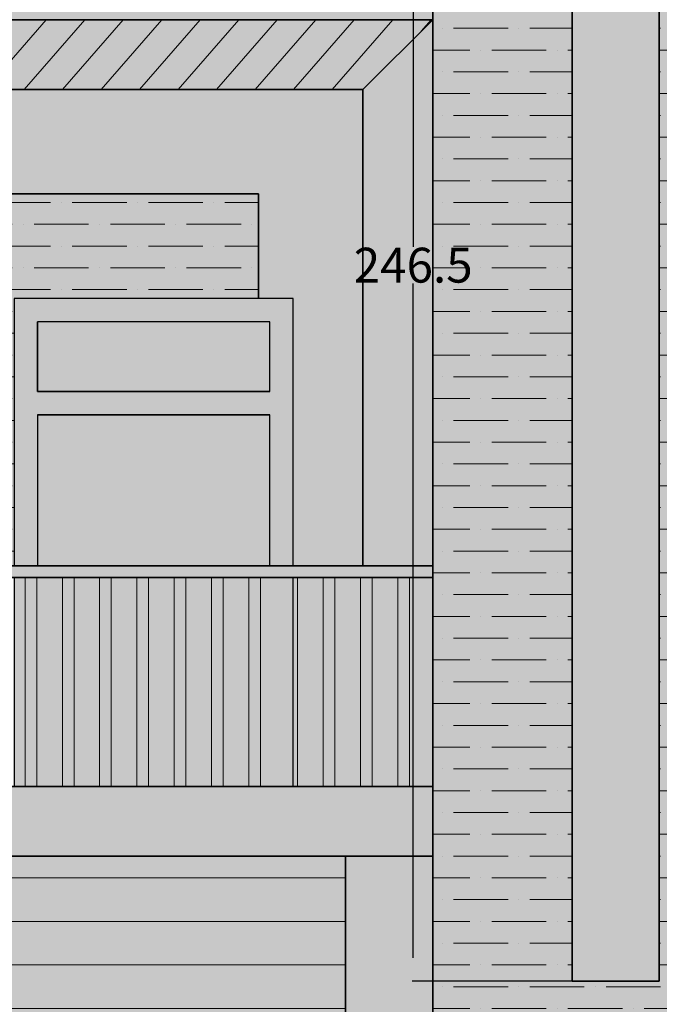
# Model space of a CAD drawing. Units: inches. Extents: x 184 to 649, y 215 to 818.
# Tile 7 of 9: x 382 to 492, y 473 to 643. Entities that reach past the tile are written whole.
import ezdxf

# ---------------------------------------------------------------- set-up
doc = ezdxf.new("R2010")
doc.units = ezdxf.units.IN
doc.header["$MEASUREMENT"] = 0
for name, color, linetype, lineweight in [('A-ANNO-DIMS', 2, 'Continuous', 18), ('A-DOOR', 4, 'Continuous', 25), ('A-ELEV', 7, 'Continuous', 35), ('A-ELEV-FILL', 9, 'Continuous', 13), ('A-ELEV-PATT', 8, 'Continuous', 13), ('A-ELEV-RAIL', 8, 'Continuous', 18)]:
    doc.layers.add(name, color=color, linetype=linetype, lineweight=lineweight)
doc.styles.get("Standard").update_dxf_attribs({"font": 'arial.ttf'})
doc.dimstyles.get("Standard").update_dxf_attribs({"dimtxt": 6, "dimasz": 4, "dimexe": 0.18, "dimexo": 0.0625, "dimgap": 0.09, "dimtad": 0, "dimtih": 1, "dimtoh": 1, "dimdec": 0, "dimzin": 0, "dimdsep": 46, "dimlunit": 3, "dimtxsty": 'Standard', "dimcen": 0.09, "dimadec": 0, "dimazin": 0, "dimtfac": 1, "dimtdec": 0, "dimtofl": 0, "dimtmove": 0, "dimatfit": 3, "dimfxl": 1, "dimtolj": 1, "dimtzin": 0, "dimarcsym": 0})

# ---------------------------------------------------------------- blocks, each defined once
blk = doc.blocks.new('DOOR-BALCONY')
for points in [[(340, 548.73), (340, 594.73), (292, 594.73), (292, 548.73)], [(336, 578.73), (336, 590.73), (296, 590.73), (296, 578.73)], [(296, 574.73), (296, 548.73)], [(336, 548.73), (336, 574.73)], [(292, 546.73), (292, 510.73), (340, 510.73), (340, 546.73)]]:
    blk.add_lwpolyline(points)
blk = doc.blocks.new('*D63')
at = {"layer": 'A-ANNO-DIMS', "color": 0, "lineweight": -2, "transparency": 16777216}
for p, q in [((476.91, 723.73), (449.44, 723.73)), ((449.62, 719.73), (449.62, 603.63)), ((449.62, 481.22), (449.62, 597.32)), ((476.91, 477.22), (449.44, 477.22))]:
    blk.add_line(p, q, dxfattribs=at)
at = {"layer": 'A-ANNO-DIMS', "color": 0, "transparency": 16777216}
for points in [[(448.96, 719.73), (450.29, 719.73), (449.62, 723.73)], [(448.96, 481.22), (450.29, 481.22), (449.62, 477.22)]]:
    blk.add_solid(points, dxfattribs=at)
at = {"layer": 'Defpoints', "color": 0, "transparency": 16777216}
for p in [(449.62, 723.73), (476.97, 723.73), (476.97, 477.22)]:
    blk.add_point(p, dxfattribs=at)
at = {"layer": 'A-ANNO-DIMS', "color": 0, "transparency": 16777216, "insert": (449.62, 600.47), "char_height": 6, "attachment_point": 5}
blk.add_mtext('\\A1;246.5', dxfattribs=at)

msp = doc.modelspace()

# ---------------------------------------------------------------- hatches: boundary and pattern name
at = {"layer": 'A-ELEV-FILL'}
h = msp.add_hatch(color=256, dxfattribs=at)
h.dxf.hatch_style = 1
h.paths.add_polyline_path([(452.9726, 369.7265), (248.9726, 369.7265), (248.9726, 246.7265), (275.9726, 246.7265), (275.9726, 328.7265), (437.9726, 328.7265), (437.9726, 246.7265), (446.6666, 246.7265), (452.9726, 282.7265)])
h.paths.add_polyline_path([(275.9726, 340.7265), (275.9726, 354.7265), (437.9726, 354.7265), (437.9726, 340.7265)], flags=16)
h.paths.add_polyline_path([(452.9726, 510.7265), (260.9726, 510.7265), (260.9726, 642.7265), (260.9726, 699.7265), (367.0226, 699.7265), (373.9381, 706.7265), (260.9726, 706.7265), (260.9726, 715.7265), (382.8295, 715.7265), (389.745, 722.7265), (260.9726, 722.7265), (260.9726, 731.7265), (398.6364, 731.7265), (405.5519, 738.7265), (260.9726, 738.7265), (260.9726, 747.7265), (414.4433, 747.7265), (421.3588, 754.7265), (260.9726, 754.7265), (260.9726, 763.7265), (430.2502, 763.7265), (437.1657, 770.7265), (260.9726, 770.7265), (260.9726, 779.7265), (446.057, 779.7265), (452.9726, 786.7265), (248.9726, 786.7265), (248.9726, 369.7265), (260.9726, 369.7265), (260.9726, 498.7265), (452.9726, 498.7265)])
h = msp.add_hatch(color=256, dxfattribs=at)
h.dxf.hatch_style = 1
h.paths.add_polyline_path([(380.9726, 453.5037), (422.2268, 453.5037), (422.2268, 474.7265), (260.9726, 474.7265), (260.9726, 369.7265), (291.9998, 369.7265), (291.9998, 453.5037), (339.9998, 453.5037), (339.9998, 369.7265), (380.9726, 369.7265)])
h.paths.add_polyline_path([(437.9726, 328.7265), (275.9726, 328.7265), (275.9726, 246.7265), (437.9726, 246.7265)])
h.paths.add_polyline_path([(581.9726, 759.7265), (521.9726, 759.7265), (521.9726, 441.2233), (581.9726, 441.2233)])
h.paths.add_polyline_path([(560.9726, 582.4749), (560.9726, 477.2233), (542.9726, 477.2233), (542.9726, 582.4749)], flags=16)
h.paths.add_polyline_path([(560.9726, 618.4749), (542.9726, 618.4749), (542.9726, 723.7265), (560.9726, 723.7265)], flags=16)
h = msp.add_hatch(color=256, dxfattribs=at)
h.dxf.hatch_style = 1
h.paths.add_polyline_path([(521.9726, 759.7265), (452.9726, 759.7265), (452.9726, 441.2233), (521.9726, 441.2233)])
h.paths.add_polyline_path([(491.9726, 477.2233), (476.9726, 477.2233), (476.9726, 723.7265), (491.9726, 723.7265)], flags=16)
h = msp.add_hatch(color=256, dxfattribs=at)
h.dxf.hatch_style = 1
h.paths.add_polyline_path([(491.9726, 723.7265), (476.9726, 723.7265), (476.9726, 477.2233), (491.9726, 477.2233)])
h = msp.add_hatch(color=256, dxfattribs=at)
h.dxf.hatch_style = 1
h.paths.add_polyline_path([(452.9726, 654.7265), (260.9726, 654.7265), (260.9726, 642.7265), (452.9726, 642.7265)])
h = msp.add_hatch(color=256, dxfattribs=at)
h.dxf.hatch_style = 1
h.paths.add_polyline_path([(440.9726, 630.7265), (260.9726, 630.7265), (260.9726, 612.7265), (422.9726, 612.7265), (422.9726, 594.7265), (428.9726, 594.7265), (428.9726, 548.7265), (440.9726, 548.7265)])
h.paths.add_polyline_path([(452.9726, 642.7265), (440.9726, 630.7265), (440.9726, 548.7265), (452.9726, 548.7265)])
h = msp.add_hatch(color=256, dxfattribs=at)
h.dxf.hatch_style = 1
h.paths.add_polyline_path([(452.9726, 642.7265), (260.9726, 642.7265), (260.9726, 630.7265), (440.9726, 630.7265)])
h = msp.add_hatch(color=256, dxfattribs=at)
h.dxf.hatch_style = 1
h.paths.add_polyline_path([(380.9726, 594.7265), (422.9726, 594.7265), (422.9726, 612.7265), (260.9726, 612.7265), (260.9726, 548.7265), (291.9998, 548.7265), (291.9998, 594.7265), (339.9998, 594.7265), (339.9998, 548.7265), (380.9726, 548.7265)])
h = msp.add_hatch(color=256, dxfattribs=at)
h.dxf.hatch_style = 1
h.paths.add_polyline_path([(339.9998, 594.7265), (291.9998, 594.7265), (291.9998, 548.7265), (295.9998, 548.7265), (295.9998, 574.7265), (335.9998, 574.7265), (335.9998, 548.7265), (339.9998, 548.7265)])
h.paths.add_polyline_path([(335.9998, 578.7265), (295.9998, 578.7265), (295.9998, 590.7265), (335.9998, 590.7265)], flags=16)
h.paths.add_polyline_path([(422.9726, 578.7265), (384.9726, 578.7265), (384.9726, 590.7265), (422.9726, 590.7265), (422.9726, 594.7265), (380.9726, 594.7265), (380.9726, 548.7265), (384.9726, 548.7265), (384.9726, 574.7265), (422.9726, 574.7265)])
h = msp.add_hatch(color=256, dxfattribs=at)
h.dxf.hatch_style = 1
h.paths.add_polyline_path([(428.9726, 594.7265), (422.9726, 594.7265), (422.9726, 590.7265), (424.9726, 590.7265), (424.9726, 578.7265), (422.9726, 578.7265), (422.9726, 574.7265), (424.9726, 574.7265), (424.9726, 548.7265), (428.9726, 548.7265)])
h = msp.add_hatch(color=256, dxfattribs=at)
h.dxf.hatch_style = 1
h.paths.add_polyline_path([(335.9998, 433.5037), (295.9998, 433.5037), (295.9998, 369.7265), (335.9998, 369.7265)])
h.paths.add_polyline_path([(335.9998, 449.5037), (295.9998, 449.5037), (295.9998, 437.5037), (335.9998, 437.5037)])
h.paths.add_polyline_path([(422.2268, 449.5037), (384.9726, 449.5037), (384.9726, 437.5037), (422.2268, 437.5037)])
h.paths.add_polyline_path([(422.2268, 433.5037), (384.9726, 433.5037), (384.9726, 369.7265), (422.2268, 369.7265)])
h.paths.add_polyline_path([(335.9998, 590.7265), (295.9998, 590.7265), (295.9998, 578.7265), (335.9998, 578.7265)])
h.paths.add_polyline_path([(335.9998, 574.7265), (295.9998, 574.7265), (295.9998, 548.7265), (335.9998, 548.7265)])
h.paths.add_polyline_path([(422.9726, 590.7265), (384.9726, 590.7265), (384.9726, 578.7265), (422.9726, 578.7265)])
h.paths.add_polyline_path([(422.9726, 574.7265), (384.9726, 574.7265), (384.9726, 548.7265), (422.9726, 548.7265)])
h = msp.add_hatch(color=256, dxfattribs=at)
h.dxf.hatch_style = 1
h.paths.add_polyline_path([(424.9726, 590.7265), (422.9726, 590.7265), (422.9726, 578.7265), (424.9726, 578.7265)])
h.paths.add_polyline_path([(424.9726, 574.7265), (422.9726, 574.7265), (422.9726, 548.7265), (424.9726, 548.7265)])
h = msp.add_hatch(color=256, dxfattribs=at)
h.dxf.hatch_style = 1
h.paths.add_polyline_path([(452.9726, 548.7265), (260.9726, 548.7265), (260.9726, 546.7265), (452.9726, 546.7265)])
h.paths.add_polyline_path([(262.9726, 546.7265), (260.9726, 546.7265), (260.9726, 510.7265), (262.9726, 510.7265)])
h.paths.add_polyline_path([(269.3864, 546.7265), (267.3864, 546.7265), (267.3864, 510.7265), (269.3864, 510.7265)])
h.paths.add_polyline_path([(275.8001, 546.7265), (273.8001, 546.7265), (273.8001, 510.7265), (275.8001, 510.7265)])
h.paths.add_polyline_path([(282.2139, 546.7265), (280.2139, 546.7265), (280.2139, 510.7265), (282.2139, 510.7265)])
h.paths.add_polyline_path([(288.6277, 546.7265), (286.6277, 546.7265), (286.6277, 510.7265), (288.6277, 510.7265)])
h.paths.add_polyline_path([(295.0415, 546.7265), (293.0415, 546.7265), (293.0415, 510.7265), (295.0415, 510.7265)])
h.paths.add_polyline_path([(301.4553, 546.7265), (299.4553, 546.7265), (299.4553, 514.7265), (301.4553, 514.7265)])
h.paths.add_polyline_path([(307.8691, 546.7265), (305.8691, 546.7265), (305.8691, 514.7265), (307.8691, 514.7265)])
h.paths.add_polyline_path([(314.2829, 546.7265), (312.2829, 546.7265), (312.2829, 514.7265), (314.2829, 514.7265)])
h.paths.add_polyline_path([(320.6967, 546.7265), (318.6967, 546.7265), (318.6967, 514.7265), (320.6967, 514.7265)])
h.paths.add_polyline_path([(327.1105, 546.7265), (325.1105, 546.7265), (325.1105, 514.7265), (327.1105, 514.7265)])
h.paths.add_polyline_path([(333.5243, 546.7265), (331.5243, 546.7265), (331.5243, 514.7265), (333.5243, 514.7265)])
h.paths.add_polyline_path([(339.9381, 546.7265), (337.9381, 546.7265), (337.9381, 510.7265), (339.9381, 510.7265)])
h.paths.add_polyline_path([(346.3519, 546.7265), (344.3519, 546.7265), (344.3519, 510.7265), (346.3519, 510.7265)])
h.paths.add_polyline_path([(352.7657, 546.7265), (350.7657, 546.7265), (350.7657, 510.7265), (352.7657, 510.7265)])
h.paths.add_polyline_path([(359.1795, 546.7265), (357.1795, 546.7265), (357.1795, 510.7265), (359.1795, 510.7265)])
h.paths.add_polyline_path([(365.5932, 546.7265), (363.5932, 546.7265), (363.5932, 510.7265), (365.5932, 510.7265)])
h.paths.add_polyline_path([(372.007, 546.7265), (370.007, 546.7265), (370.007, 510.7265), (372.007, 510.7265)])
h.paths.add_polyline_path([(378.4208, 546.7265), (376.4208, 546.7265), (376.4208, 510.7265), (378.4208, 510.7265)])
h.paths.add_polyline_path([(384.8346, 546.7265), (382.8346, 546.7265), (382.8346, 510.7265), (384.8346, 510.7265)])
h.paths.add_polyline_path([(391.2484, 546.7265), (389.2484, 546.7265), (389.2484, 514.7265), (391.2484, 514.7265)])
h.paths.add_polyline_path([(397.6622, 546.7265), (395.6622, 546.7265), (395.6622, 514.7265), (397.6622, 514.7265)])
h.paths.add_polyline_path([(404.076, 546.7265), (402.076, 546.7265), (402.076, 514.7265), (404.076, 514.7265)])
h.paths.add_polyline_path([(410.4898, 546.7265), (408.4898, 546.7265), (408.4898, 514.7265), (410.4898, 514.7265)])
h.paths.add_polyline_path([(416.9036, 546.7265), (414.9036, 546.7265), (414.9036, 514.7265), (416.9036, 514.7265)])
h.paths.add_polyline_path([(423.3174, 546.7265), (421.3174, 546.7265), (421.3174, 514.7265), (423.3174, 514.7265)])
h.paths.add_polyline_path([(423.3174, 514.7265), (421.3174, 514.7265), (421.3174, 510.7265), (423.3174, 510.7265)])
h.paths.add_polyline_path([(416.9036, 514.7265), (414.9036, 514.7265), (414.9036, 510.7265), (416.9036, 510.7265)])
h.paths.add_polyline_path([(410.4898, 514.7265), (408.4898, 514.7265), (408.4898, 510.7265), (410.4898, 510.7265)])
h.paths.add_polyline_path([(404.076, 514.7265), (402.076, 514.7265), (402.076, 510.7265), (404.076, 510.7265)])
h.paths.add_polyline_path([(397.6622, 514.7265), (395.6622, 514.7265), (395.6622, 510.7265), (397.6622, 510.7265)])
h.paths.add_polyline_path([(391.2484, 514.7265), (389.2484, 514.7265), (389.2484, 510.7265), (391.2484, 510.7265)])
h.paths.add_polyline_path([(448.9726, 546.7265), (446.9726, 546.7265), (446.9726, 510.7265), (448.9726, 510.7265)])
h.paths.add_polyline_path([(442.5588, 546.7265), (440.5588, 546.7265), (440.5588, 510.7265), (442.5588, 510.7265)])
h.paths.add_polyline_path([(436.145, 546.7265), (434.145, 546.7265), (434.145, 510.7265), (436.145, 510.7265)])
h.paths.add_polyline_path([(429.7312, 546.7265), (428.9726, 546.7265), (428.9726, 510.7265), (429.7312, 510.7265)])
h.paths.add_polyline_path([(301.4553, 514.7265), (299.4553, 514.7265), (299.4553, 510.7265), (301.4553, 510.7265)])
h.paths.add_polyline_path([(307.8691, 514.7265), (305.8691, 514.7265), (305.8691, 510.7265), (307.8691, 510.7265)])
h.paths.add_polyline_path([(314.2829, 514.7265), (312.2829, 514.7265), (312.2829, 510.7265), (314.2829, 510.7265)])
h.paths.add_polyline_path([(320.6967, 514.7265), (318.6967, 514.7265), (318.6967, 510.7265), (320.6967, 510.7265)])
h.paths.add_polyline_path([(327.1105, 514.7265), (325.1105, 514.7265), (325.1105, 510.7265), (327.1105, 510.7265)])
h.paths.add_polyline_path([(333.5243, 514.7265), (331.5243, 514.7265), (331.5243, 510.7265), (333.5243, 510.7265)])
h = msp.add_hatch(color=256, dxfattribs=at)
h.dxf.hatch_style = 1
h.paths.add_polyline_path([(382.8346, 546.7265), (380.9726, 546.7265), (380.9726, 510.7265), (382.8346, 510.7265)])
h.paths.add_polyline_path([(421.3174, 514.7265), (416.9036, 514.7265), (416.9036, 510.7265), (421.3174, 510.7265)])
h.paths.add_polyline_path([(414.9036, 514.7265), (410.4898, 514.7265), (410.4898, 510.7265), (414.9036, 510.7265)])
h.paths.add_polyline_path([(408.4898, 514.7265), (404.076, 514.7265), (404.076, 510.7265), (408.4898, 510.7265)])
h.paths.add_polyline_path([(402.076, 514.7265), (397.6622, 514.7265), (397.6622, 510.7265), (402.076, 510.7265)])
h.paths.add_polyline_path([(395.6622, 514.7265), (391.2484, 514.7265), (391.2484, 510.7265), (395.6622, 510.7265)])
h.paths.add_polyline_path([(389.2484, 514.7265), (384.9726, 514.7265), (384.9726, 546.7265), (384.8346, 546.7265), (384.8346, 510.7265), (389.2484, 510.7265)])
h.paths.add_polyline_path([(293.0415, 546.7265), (291.9998, 546.7265), (291.9998, 510.7265), (293.0415, 510.7265)], flags=16)
h.paths.add_polyline_path([(299.4553, 514.7265), (295.9998, 514.7265), (295.9998, 546.7265), (295.0415, 546.7265), (295.0415, 510.7265), (299.4553, 510.7265)], flags=16)
h.paths.add_polyline_path([(337.9381, 546.7265), (335.9998, 546.7265), (335.9998, 514.7265), (333.5243, 514.7265), (333.5243, 510.7265), (337.9381, 510.7265)], flags=17)
h.paths.add_polyline_path([(339.9998, 546.7265), (339.9381, 546.7265), (339.9381, 510.7265), (339.9998, 510.7265)])
h = msp.add_hatch(color=256, dxfattribs=at)
h.dxf.hatch_style = 1
h.paths.add_polyline_path([(417.6041, 354.7265), (411.9199, 354.7265), (411.9199, 340.7265), (417.6041, 340.7265)])
h.paths.add_polyline_path([(409.9199, 354.7265), (404.2357, 354.7265), (404.2357, 340.7265), (409.9199, 340.7265)])
h.paths.add_polyline_path([(402.2357, 354.7265), (396.5515, 354.7265), (396.5515, 340.7265), (402.2357, 340.7265)])
h.paths.add_polyline_path([(394.5515, 354.7265), (388.8673, 354.7265), (388.8673, 340.7265), (394.5515, 340.7265)])
h.paths.add_polyline_path([(333.0778, 354.7265), (327.3936, 354.7265), (327.3936, 340.7265), (333.0778, 340.7265)])
h.paths.add_polyline_path([(325.3936, 354.7265), (319.7094, 354.7265), (319.7094, 340.7265), (325.3936, 340.7265)])
h.paths.add_polyline_path([(317.7094, 354.7265), (312.0252, 354.7265), (312.0252, 340.7265), (317.7094, 340.7265)])
h.paths.add_polyline_path([(310.0252, 354.7265), (304.341, 354.7265), (304.341, 340.7265), (310.0252, 340.7265)])
h.paths.add_polyline_path([(302.341, 354.7265), (296.6568, 354.7265), (296.6568, 340.7265), (302.341, 340.7265)])
h.paths.add_polyline_path([(421.3174, 546.7265), (416.9036, 546.7265), (416.9036, 514.7265), (421.3174, 514.7265)])
h.paths.add_polyline_path([(414.9036, 546.7265), (410.4898, 546.7265), (410.4898, 514.7265), (414.9036, 514.7265)])
h.paths.add_polyline_path([(402.076, 546.7265), (397.6622, 546.7265), (397.6622, 514.7265), (402.076, 514.7265)])
h.paths.add_polyline_path([(395.6622, 546.7265), (391.2484, 546.7265), (391.2484, 514.7265), (395.6622, 514.7265)])
h.paths.add_polyline_path([(389.2484, 546.7265), (384.9726, 546.7265), (384.9726, 514.7265), (389.2484, 514.7265)])
h.paths.add_polyline_path([(408.4898, 546.7265), (404.076, 546.7265), (404.076, 514.7265), (408.4898, 514.7265)])
h.paths.add_polyline_path([(335.9998, 546.7265), (333.5243, 546.7265), (333.5243, 514.7265), (335.9998, 514.7265)])
h.paths.add_polyline_path([(331.5243, 546.7265), (327.1105, 546.7265), (327.1105, 514.7265), (331.5243, 514.7265)])
h.paths.add_polyline_path([(325.1105, 546.7265), (320.6967, 546.7265), (320.6967, 514.7265), (325.1105, 514.7265)])
h.paths.add_polyline_path([(318.6967, 546.7265), (314.2829, 546.7265), (314.2829, 514.7265), (318.6967, 514.7265)])
h.paths.add_polyline_path([(312.2829, 546.7265), (307.8691, 546.7265), (307.8691, 514.7265), (312.2829, 514.7265)])
h.paths.add_polyline_path([(305.8691, 546.7265), (301.4553, 546.7265), (301.4553, 514.7265), (305.8691, 514.7265)])
h.paths.add_polyline_path([(299.4553, 546.7265), (295.9998, 546.7265), (295.9998, 514.7265), (299.4553, 514.7265)])
h = msp.add_hatch(color=256, dxfattribs=at)
h.dxf.hatch_style = 1
h.paths.add_polyline_path([(427.7312, 546.7265), (424.9726, 546.7265), (424.9726, 514.7265), (423.3174, 514.7265), (423.3174, 510.7265), (427.7312, 510.7265)])
h = msp.add_hatch(color=256, dxfattribs=at)
h.dxf.hatch_style = 1
h.paths.add_polyline_path([(428.9726, 546.7265), (424.9726, 546.7265), (424.9726, 514.7265), (423.3174, 514.7265), (423.3174, 510.7265), (428.9726, 510.7265)])
h = msp.add_hatch(color=256, dxfattribs=at)
h.dxf.hatch_style = 1
h.paths.add_polyline_path([(424.9726, 546.7265), (423.3174, 546.7265), (423.3174, 514.7265), (424.9726, 514.7265)])
h = msp.add_hatch(color=256, dxfattribs=at)
h.dxf.hatch_style = 1
h.paths.add_polyline_path([(452.9726, 546.7265), (448.9726, 546.7265), (448.9726, 510.7265), (452.9726, 510.7265)])
h.paths.add_polyline_path([(446.9726, 546.7265), (442.5588, 546.7265), (442.5588, 510.7265), (446.9726, 510.7265)])
h.paths.add_polyline_path([(440.5588, 546.7265), (437.9726, 546.7265), (437.9726, 510.7265), (440.5588, 510.7265)])
h.paths.add_polyline_path([(437.9726, 546.7265), (436.145, 546.7265), (436.145, 510.7265), (437.9726, 510.7265)])
h.paths.add_polyline_path([(434.145, 546.7265), (429.7312, 546.7265), (429.7312, 510.7265), (434.145, 510.7265)])
h = msp.add_hatch(color=256, dxfattribs=at)
h.dxf.hatch_style = 1
h.paths.add_polyline_path([(437.9726, 498.7265), (260.9726, 498.7265), (260.9726, 474.7265), (422.2268, 474.7265), (422.2268, 453.5037), (428.9726, 453.5037), (428.9726, 417.0753), (445.4726, 417.0753), (445.4726, 437.9607), (437.9726, 437.9607)])
h = msp.add_hatch(color=256, dxfattribs=at)
h.dxf.hatch_style = 1
h.paths.add_polyline_path([(452.9726, 498.7265), (437.9726, 498.7265), (437.9726, 437.9607), (452.9726, 441.2233)])
at = {"layer": 'A-ELEV-PATT'}
h = msp.add_hatch(dxfattribs=at)
h.set_pattern_fill('ANSI36', color=256, scale=30, angle=135)
h.paths.add_polyline_path([(521.9726, 759.7265), (452.9726, 759.7265), (452.9726, 441.2233), (521.9726, 441.2233)])
h.paths.add_polyline_path([(476.9726, 723.7265), (491.9726, 723.7265), (491.9726, 477.2233), (476.9726, 477.2233)], flags=16)
h = msp.add_hatch(dxfattribs=at)
h.set_pattern_fill('ANSI31', color=256, scale=40, angle=4)
h.paths.add_polyline_path([(452.9726, 642.7265), (260.9726, 642.7265), (260.9726, 630.7265), (440.9726, 630.7265)])
h = msp.add_hatch(dxfattribs=at)
h.set_pattern_fill('ANSI36', color=256, scale=30, angle=135)
h.paths.add_polyline_path([(380.9726, 594.7265), (422.9726, 594.7265), (422.9726, 612.7265), (260.9726, 612.7265), (260.9726, 548.7265), (291.9998, 548.7265), (291.9998, 594.7265), (339.9998, 594.7265), (339.9998, 548.7265), (380.9726, 548.7265)])
h = msp.add_hatch(dxfattribs=at)
h.set_pattern_fill('ANSI31', color=256, scale=60, angle=135)
h.paths.add_polyline_path([(437.9726, 498.7265), (260.9726, 498.7265), (260.9726, 369.7265), (291.9998, 369.7265), (291.9998, 453.5037), (339.9998, 453.5037), (339.9998, 369.7265), (380.9726, 369.7265), (380.9726, 453.5037), (428.9726, 453.5037), (428.9726, 417.0753), (445.4726, 417.0753), (445.4726, 437.9607), (437.9726, 437.9607)])

# ---------------------------------------------------------------- linework, layer by layer
at = {"layer": 'A-ELEV'}
for p, q in [((452.9726, 441.2233), (452.9726, 759.7265)), ((476.9726, 477.2233), (476.9726, 723.7265)), ((491.9726, 477.2233), (491.9726, 723.7265)), ((452.9726, 642.7265), (260.9726, 642.7265)), ((440.9726, 630.7265), (452.9726, 642.7265)), ((440.9726, 630.7265), (260.9726, 630.7265)), ((440.9726, 548.7265), (440.9726, 630.7265)), ((422.9726, 612.7265), (260.9726, 612.7265)), ((422.9726, 594.7265), (422.9726, 612.7265)), ((384.9726, 590.7265), (384.9726, 578.7265)), ((384.9726, 578.7265), (424.9726, 578.7265)), ((424.9726, 574.7265), (384.9726, 574.7265)), ((452.9726, 548.7265), (260.9726, 548.7265)), ((452.9726, 546.7265), (260.9726, 546.7265)), ((452.9726, 510.7265), (260.9726, 510.7265)), ((452.9726, 498.7265), (260.9726, 498.7265)), ((437.9726, 437.9607), (437.9726, 498.7265)), ((476.9726, 477.2233), (491.9726, 477.2233))]:
    msp.add_line(p, q, dxfattribs=at)
at = {"layer": 'A-ELEV-RAIL'}
for p, q in [((382.8346, 510.7265), (382.8346, 546.7265)), ((384.8346, 510.7265), (384.8346, 546.7265)), ((389.2484, 510.7265), (389.2484, 546.7265)), ((391.2484, 510.7265), (391.2484, 546.7265)), ((395.6622, 510.7265), (395.6622, 546.7265)), ((397.6622, 510.7265), (397.6622, 546.7265)), ((402.076, 510.7265), (402.076, 546.7265)), ((404.076, 510.7265), (404.076, 546.7265)), ((408.4898, 510.7265), (408.4898, 546.7265)), ((410.4898, 510.7265), (410.4898, 546.7265)), ((414.9036, 510.7265), (414.9036, 546.7265)), ((416.9036, 510.7265), (416.9036, 546.7265)), ((421.3174, 510.7265), (421.3174, 546.7265)), ((423.3174, 510.7265), (423.3174, 546.7265)), ((429.7312, 510.7265), (429.7312, 546.7265)), ((434.145, 510.7265), (434.145, 546.7265)), ((436.145, 510.7265), (436.145, 546.7265)), ((440.5588, 510.7265), (440.5588, 546.7265)), ((442.5588, 510.7265), (442.5588, 546.7265)), ((446.9726, 510.7265), (446.9726, 546.7265)), ((448.9726, 510.7265), (448.9726, 546.7265))]:
    msp.add_line(p, q, dxfattribs=at)

# ---------------------------------------------------------------- block references
at = {"layer": 'A-DOOR'}
msp.add_blockref('DOOR-BALCONY', (88.9728, 0), dxfattribs=at)

# ---------------------------------------------------------------- dimensions: what is measured, and where the dimension line sits
at = {"layer": 'A-ANNO-DIMS'}
dim = msp.add_linear_dim(base=(449.6226, 723.7265), p1=(476.9726, 477.2233), p2=(476.9726, 723.7265), angle=90, dimstyle='Standard', override={"dimdec": 1, "dimlfac": 1, "dimrnd": 0, "dimzin": 0, "dimdsep": 46, "dimlunit": 2}, dxfattribs=at)
dim.commit()
dim.dimension.update_dxf_attribs({"geometry": '*D63', "text_midpoint": (449.6226, 600.4749)})

doc.saveas('drawing.dxf')
